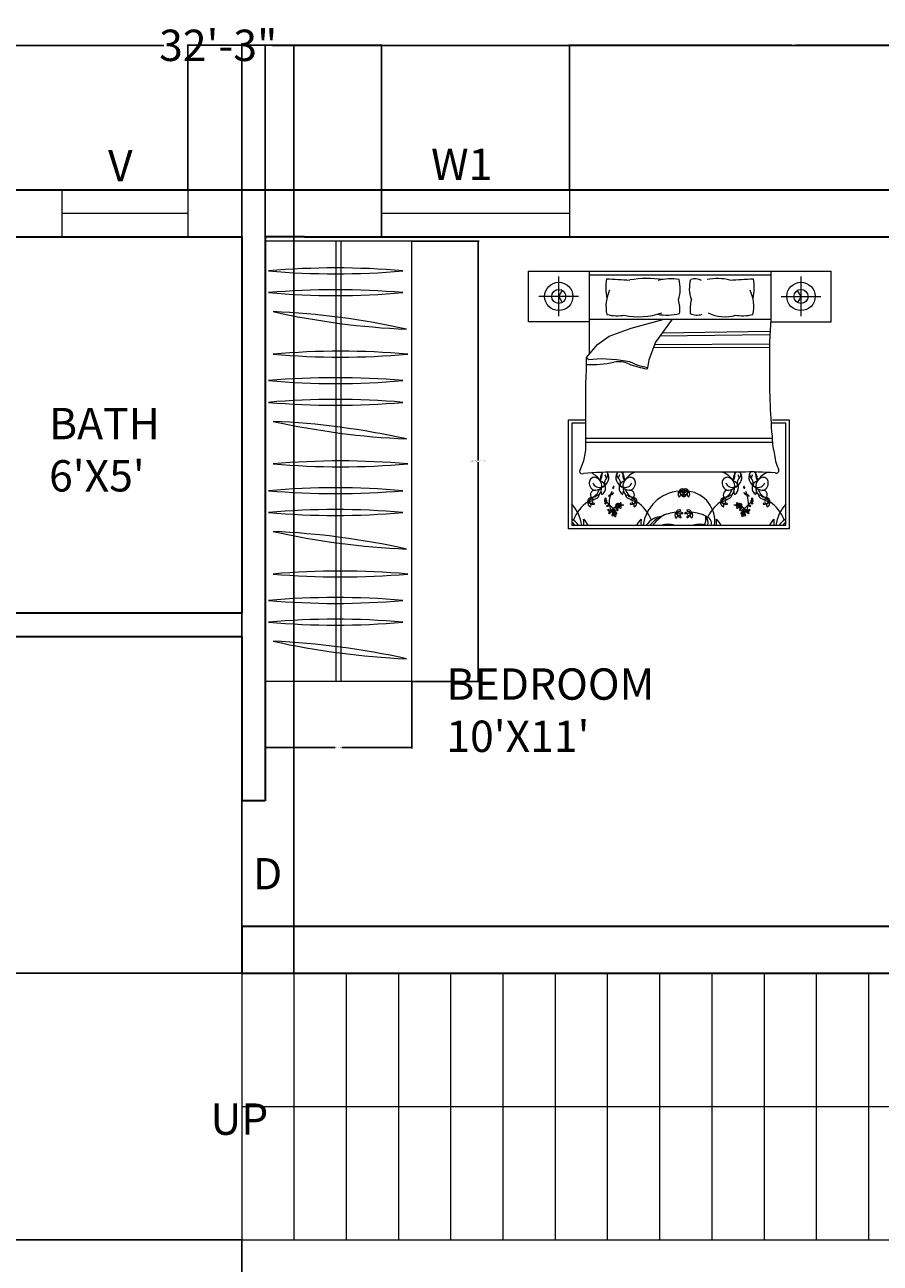
# Model space of a CAD drawing. Units: inches. Extents: x -4347 to -3836, y 955 to 1521.
# Tile 10 of 11: x -4162 to -3998, y 1284 to 1521. Entities that reach past the tile are written whole.
import ezdxf

# ---------------------------------------------------------------- set-up
doc = ezdxf.new("R2010")
doc.units = ezdxf.units.IN
doc.header["$MEASUREMENT"] = 0
for name, color, linetype, lineweight in [('A-ANNO-DIMS', 2, 'Continuous', 18), ('A-ANNO-SYMB', 7, 'Continuous', 18), ('A-ANNO-TEXT', 7, 'Continuous', 18), ('A-AREA-IDEN', 7, 'Continuous', 18), ('A-FLOR-STRS', 7, 'Continuous', 18), ('A-FURN', 8, 'Continuous', 13), ('A-GLAZ', 4, 'Continuous', 18), ('A-WALL', 7, 'Continuous', 35)]:
    doc.layers.add(name, color=color, linetype=linetype, lineweight=lineweight)
doc.styles.get("Standard").update_dxf_attribs({"font": 'arial.ttf'})
doc.dimstyles.get("Standard").update_dxf_attribs({"dimtxt": 0.18, "dimasz": 0.18, "dimexe": 0.18, "dimexo": 0.0625, "dimgap": 0.09, "dimtad": 0, "dimtih": 1, "dimtoh": 1, "dimdec": 0, "dimzin": 0, "dimdsep": 46, "dimlunit": 3, "dimtxsty": 'Standard', "dimcen": 0.09, "dimadec": 0, "dimazin": 0, "dimtfac": 1, "dimtdec": 0, "dimtofl": 0, "dimtmove": 0, "dimatfit": 3, "dimfxl": 1, "dimtolj": 1, "dimtzin": 0, "dimarcsym": 0})

# ---------------------------------------------------------------- blocks, each defined once
blk = doc.blocks.new('*D1')
at = {"layer": 'A-ANNO-DIMS', "color": 0, "lineweight": -2, "transparency": 16777216}
for p, q in [((-4318.58, 1489.85), (-4318.58, 1517.61)), ((-4318.4, 1517.43), (-4135.47, 1517.43)), ((-3931.76, 1517.43), (-4114.69, 1517.43)), ((-3931.58, 1489.85), (-3931.58, 1517.61))]:
    blk.add_line(p, q, dxfattribs=at)
at = {"layer": 'A-ANNO-DIMS', "color": 0, "transparency": 16777216}
for points in [[(-4318.4, 1517.46), (-4318.4, 1517.4), (-4318.58, 1517.43)], [(-3931.76, 1517.46), (-3931.76, 1517.4), (-3931.58, 1517.43)]]:
    blk.add_solid(points, dxfattribs=at)
at = {"layer": 'Defpoints', "color": 0, "transparency": 16777216}
for p in [(-3931.58, 1517.43), (-4318.58, 1489.79), (-3931.58, 1489.79)]:
    blk.add_point(p, dxfattribs=at)
at = {"layer": 'A-ANNO-DIMS', "color": 0, "transparency": 16777216, "insert": (-4125.08, 1517.43), "char_height": 6, "attachment_point": 5}
blk.add_mtext('\\A1;32\'-3"', dxfattribs=at)
blk = doc.blocks.new('BED-DOUBLE-WITH-NIGHTSTANDS')
for p, q in [((0, 49.3), (57.97, 49.3)), ((5.8, 40.68), (5.8, 48.26)), ((11.59, 49.3), (11.59, 33.39)), ((46.38, 48.56), (11.59, 48.56)), ((52.18, 40.68), (52.18, 48.26)), ((9.59, 44.47), (2.01, 44.47)), ((48.39, 44.47), (55.96, 44.47)), ((11.59, 40.14), (46.38, 40.14)), ((15.42, 36.89), (19.65, 38.42)), ((19.65, 38.42), (25.97, 40.14)), ((27.52, 40.14), (24.34, 35.72)), ((13.19, 35.25), (15.42, 36.89)), ((24.34, 35.72), (23.05, 32.32)), ((46.2, 37.14), (25.15, 36.84)), ((46.22, 37.73), (25.58, 37.44)), ((11.08, 32.79), (13.19, 35.25)), ((46.17, 34.72), (23.93, 34.63)), ((46.17, 35.31), (24.16, 35.23)), ((11.55, 32.32), (11.08, 32.79)), ((13.89, 32.55), (11.55, 32.32)), ((16.83, 32.32), (13.89, 32.55)), ((19.41, 31.96), (16.83, 32.32)), ((20.94, 31.26), (19.41, 31.96)), ((22.82, 30.79), (20.94, 31.26)), ((23.05, 32.32), (22.82, 30.79)), ((7.65, 20.88), (10.93, 20.88)), ((7.65, 0), (7.65, 20.88)), ((10.93, 20.21), (8.32, 20.21)), ((8.32, 20.21), (8.32, 0.67)), ((49.25, 20.21), (46.69, 20.21)), ((46.7, 20.88), (49.92, 20.88)), ((49.25, 0.67), (49.25, 20.21)), ((49.92, 20.88), (49.92, 0)), ((46.64, 17.27), (10.93, 17.27)), ((46.7, 16.54), (10.93, 16.54)), ((40.76, 10.85), (17.22, 10.85)), ((14.04, 6.55), (13.91, 7.2)), ((18.09, 6.55), (18.22, 7.2)), ((39.48, 6.55), (39.35, 7.2)), ((43.53, 6.55), (43.66, 7.2)), ((8.32, 0.67), (49.25, 0.67)), ((49.92, 0), (7.65, 0))]:
    blk.add_line(p, q)
for points in [[(11.59, 39.64), (0, 39.64), (0, 49.3)], [(46.38, 49.3), (46.38, 39.64), (57.97, 39.64), (57.97, 49.3)], [(5.8, 44.47), (6.47, 45.64)], [(52.18, 44.47), (51.5, 45.64)], [(5.8, 44.47), (6.47, 43.3)], [(52.18, 44.47), (51.5, 43.3)]]:
    blk.add_lwpolyline(points)
for points in [[(14.92, 47.86, 0.074897), (15, 44.07, -0.472817)], [(28.72, 43.86, 0.14099), (28.83, 47.72, 0.235245)], [(31.19, 43.86, -0.14099), (31.08, 47.72, -0.235245)], [(43.05, 47.86, -0.074897), (42.98, 44.07, 0.472817)], [(10.95, 27.48, 0.001242), (10.93, 16.48, -0.127202), (9.76, 10.99)], [(46.63, 17.72, 0.056112), (47.05, 14.53, 0.095341), (47.86, 11.46)]]:
    blk.add_lwpolyline(points, format="xyb")
for centre, radius in [((5.8, 44.47), 2.71), ((5.8, 44.47), 1.35), ((52.18, 44.47), 2.71), ((52.18, 44.47), 1.35), ((16.42, 2.89), 0.148), ((17.39, 4.45), 0.148), ((40.18, 4.45), 0.148), ((41.15, 2.89), 0.148)]:
    blk.add_circle(centre, radius)
for centre, radius, start, end in [((46.88, 599.58), 552.65, 266.6852, 267.1498), ((22.87, 26.88), 21.03, 82.2196, 99.497), ((27.31, 37.51), 10.33, 81.5249, 103.96), ((31.87, 44.97), 2.87, 63.3437, 106.1026), ((36.17, 37.71), 10.19, 76.3427, 101.1841), ((11.09, 599.58), 552.65, 272.8502, 273.3148), ((22.31, 42.55), 7.47, 155.1316, 191.7583), ((35.66, 42.55), 7.47, 348.2417, 24.8684), ((21.88, 41.92), 7.1, 354.0129, 15.8293), ((38.03, 41.92), 7.1, 164.1707, 185.9871), ((16.99, 48.54), 7.77, 255.1039, 281.0369), ((21.08, 54.06), 13.48, 258.0397, 289.2615), ((26.54, 51.12), 10.22, 259.8617, 283.6238), ((32.26, 43.97), 3.07, 245.0183, 288.5407), ((37.63, 47.96), 7.38, 243.8761, 286.1746), ((40.98, 48.54), 7.77, 258.9631, 284.8961), ((150.31, 33.06), 104.17, 176.1, 180.9282), ((-42.08, 31.34), 53.18, 355.8294, 1.553), ((12.07, 53.32), 21.88, 267.4519, 281.3392), ((17.3, 27.24), 4.72, 66.2616, 101.3392), ((26.84, 52.7), 22.48, 250.1194, 259.3383), ((182.02, 29.27), 135.88, 179.1145, 184.8735), ((22.69, 30.74), 0.14, 268.8623, 19.7536), ((10.3, 11.03), 0.535, 183.98, 297.3412), ((16.53, -49.5), 60.35, 89.3433, 95.6887), ((12.63, 8.87), 0.979, 84.4856, 181.0538), ((10.07, 6.77), 4.39, 33.6671, 63.2997), ((12.33, 8.15), 1.74, 355.2933, 76.921), ((15.95, 9.38), 2.24, 145.785, 184.7304), ((11.68, 10.42), 2.4, 328.8218, 9.1554), ((14.66, 10.21), 0.698, 120.0293, 142.325), ((13.54, 9.8), 1.85, 289.2822, 29.1751), ((15.73, 8.81), 1.19, 131.5653, 195.1471), ((13.26, 9.46), 1.67, 7.436, 29.9149), ((14.36, 10.35), 0.867, 311.5653, 23.8354), ((14.66, 10.21), 0.698, 44.4517, 63.558), ((18.58, 9.8), 1.85, 150.8249, 250.7178), ((17.76, 10.35), 0.867, 156.1646, 228.4347), ((17.47, 10.21), 0.698, 113.229, 135.5483), ((16.4, 8.81), 1.19, 344.8529, 48.4347), ((18.86, 9.46), 1.67, 150.0851, 172.564), ((17.47, 10.21), 0.698, 37.675, 66.7144), ((16.17, 9.38), 2.24, 355.2696, 34.215), ((20.44, 10.42), 2.4, 169.7133, 211.1782), ((19.8, 8.15), 1.74, 103.079, 184.7067), ((22.05, 6.77), 4.39, 111.4941, 146.3329), ((19.5, 8.87), 0.979, 358.9462, 95.5144), ((38.07, 8.87), 0.979, 84.4856, 181.0538), ((35.52, 6.77), 4.39, 33.6671, 68.5059), ((37.77, 8.15), 1.74, 355.2933, 76.921), ((41.4, 9.38), 2.24, 145.785, 184.7304), ((37.13, 10.42), 2.4, 328.8218, 10.2867), ((40.1, 10.21), 0.698, 113.2856, 142.325), ((38.99, 9.8), 1.85, 289.2822, 29.1751), ((41.17, 8.81), 1.19, 131.5653, 195.1471), ((38.71, 9.46), 1.67, 7.436, 29.9149), ((40.1, 10.21), 0.698, 44.4517, 66.7144), ((39.81, 10.35), 0.867, 311.5653, 23.8354), ((42.53, -45.54), 56.41, 85.2402, 91.8035), ((44.03, 9.8), 1.85, 150.8249, 250.7178), ((43.21, 10.35), 0.867, 156.1646, 228.4347), ((42.91, 10.21), 0.698, 106.6343, 135.5483), ((41.84, 8.81), 1.19, 344.8529, 48.4347), ((44.31, 9.46), 1.67, 150.0851, 172.564), ((42.91, 10.21), 0.698, 37.675, 72.5814), ((41.62, 9.38), 2.24, 355.2696, 34.215), ((45.89, 10.42), 2.4, 169.249, 211.1782), ((45.24, 8.15), 1.74, 103.079, 184.7067), ((47.5, 6.77), 4.39, 113.6453, 146.3329), ((44.94, 8.87), 0.979, 358.9462, 95.5144), ((47.42, 11.17), 0.528, 246.5219, 33.8264), ((13.03, 8.73), 1.39, 174.9449, 262.8857), ((12.71, 6.5), 0.87, 80.264, 250.8688), ((13.57, 9.26), 1.35, 201.5819, 291.4221), ((10.99, 8.42), 2.74, 301.2614, 341.7045), ((12.79, 9.04), 1.68, 272.3591, 324.0401), ((10.96, 8.2), 3.11, 326.2883, 356.5076), ((13.32, 7.8), 1.44, 299.9085, 73.1337), ((15.95, 9.38), 2.24, 212.7011, 216.3445), ((14.23, 8.4), 0.36, 257.3041, 15.1471), ((20.25, 4.94), 4.8, 153.0032, 159.8941), ((16.23, 7.86), 0.112, 102.7051, 280.4384), ((16.22, 7.93), 0.182, 280.4384, 100.4136), ((18.81, 7.8), 1.44, 106.8663, 240.0915), ((17.89, 8.4), 0.36, 164.8529, 282.6959), ((16.17, 9.38), 2.24, 323.6555, 327.2989), ((19.34, 9.04), 1.68, 215.9599, 267.6409), ((18.55, 9.26), 1.35, 248.5779, 338.4181), ((21.17, 8.2), 3.11, 183.4924, 213.7117), ((21.14, 8.42), 2.74, 198.2955, 238.7386), ((19.1, 8.73), 1.39, 277.1143, 5.0551), ((19.41, 6.5), 0.87, 289.1312, 99.736), ((29.44, -0.35), 7.57, 94.4623, 172.255), ((29.47, 6.63), 0.84, 137.7873, 219.1145), ((28.52, 6.66), 0.632, 298.5391, 58.3627), ((29.45, 7.02), 0.628, 63.0274, 163.8037), ((28.82, 8.49), 1.29, 271.4585, 315.3727), ((29.34, 6.11), 1.2, 45.5411, 114.3101), ((30.43, 12.25), 5.3, 252.593, 267.2582), ((29.47, 7.17), 0.619, 177.7585, 283.852), ((30.66, 7.82), 1.91, 198.9159, 238.011), ((30.16, 6.11), 1.2, 65.6899, 134.4589), ((29.07, 12.25), 5.3, 272.7418, 287.407), ((30.05, 7.02), 0.628, 16.1963, 116.9726), ((30.69, 8.49), 1.29, 224.6273, 268.5415), ((28.84, 7.82), 1.91, 301.989, 341.0841), ((30.03, 7.17), 0.619, 256.148, 2.2415), ((30.99, 6.66), 0.632, 121.6373, 241.4609), ((30.03, 6.63), 0.84, 320.8855, 42.2127), ((29.82, 1.4), 5.86, 352.8636, 81.8197), ((38.47, 8.73), 1.39, 174.9449, 262.8857), ((38.16, 6.5), 0.87, 80.264, 250.8688), ((39.02, 9.26), 1.35, 201.5819, 291.4221), ((36.43, 8.42), 2.74, 301.2614, 341.7045), ((38.23, 9.04), 1.68, 272.3591, 324.0401), ((36.4, 8.2), 3.11, 326.2883, 356.5076), ((38.76, 7.8), 1.44, 299.9085, 73.1337), ((41.4, 9.38), 2.24, 212.7011, 216.3445), ((39.68, 8.4), 0.36, 257.3041, 15.1471), ((41.35, 7.93), 0.182, 79.5864, 259.5616), ((41.34, 7.86), 0.112, 259.5616, 77.2949), ((37.32, 4.94), 4.8, 20.1059, 26.9968), ((44.25, 7.8), 1.44, 106.8663, 240.0915), ((43.34, 8.4), 0.36, 164.8529, 282.6959), ((41.62, 9.38), 2.24, 323.6555, 327.2989), ((44.78, 9.04), 1.68, 215.9599, 267.6409), ((44, 9.26), 1.35, 248.5779, 338.4181), ((46.61, 8.2), 3.11, 183.4924, 213.7117), ((46.58, 8.42), 2.74, 198.2955, 238.7386), ((44.54, 8.73), 1.39, 277.1143, 5.0551), ((44.86, 6.5), 0.87, 289.1312, 99.736), ((15.64, -1.1), 7.57, 124.3865, 158.5908), ((12.18, 4.97), 0.84, 167.7115, 249.0387), ((11.97, 5.3), 0.628, 92.9516, 193.728), ((10.69, 6.25), 1.29, 301.3827, 345.2969), ((12.34, 4.45), 1.2, 75.4653, 144.2343), ((10.22, 10.32), 5.3, 282.5173, 297.1824), ((11.35, 4.52), 0.632, 328.4633, 88.2869), ((12.62, 6.59), 1.91, 228.8402, 267.9352), ((11.91, 5.44), 0.619, 207.6827, 313.7762), ((12.53, 5.56), 0.533, 63.9755, 143.2681), ((12.28, 5.05), 0.0819, 313.7762, 249.7183), ((12.5, 6.76), 1.09, 265.969, 344.3045), ((12.55, 4.82), 0.0457, 101.4834, 217.9409), ((12.56, 4.77), 0.094, 267.9352, 101.4834), ((13.67, 5.32), 1.16, 96.1662, 141.5825), ((14.73, 5.55), 0.246, 101.5637, 142.6358), ((14.52, 5.33), 0.148, 273.2768, 86.7232), ((14.73, 5.05), 0.244, 217.7621, 259.0403), ((14.7, 5.47), 0.141, 91.1081, 181.8675), ((14.99, 5.38), 0.448, 203.4276, 227.6104), ((14.53, 5.75), 0.355, 288.7263, 352.5032), ((14.85, 5.18), 0.305, 80.3487, 133.6538), ((14.79, 5.43), 0.242, 229.7889, 317.6792), ((14.52, 4.92), 0.343, 355.053, 68.3618), ((14.79, 4.86), 0.483, 83.0852, 105.7171), ((14.77, 5.73), 0.114, 345.2356, 144.9248), ((14.75, 4.9), 0.113, 232.4737, 355.053), ((11.44, 0.86), 5.5, 43.1541, 52.0459), ((14.88, 5.36), 0.127, 317.6792, 80.3487), ((15.59, 6.13), 0.304, 101.3256, 154.4621), ((15.15, 7.16), 0.916, 280.2588, 300.656), ((15.36, 7.9), 1.63, 268.3264, 277.1302), ((20.25, 4.94), 4.8, 163.5842, 183.8277), ((14.95, 7.16), 0.931, 308.2101, 316.3071), ((15.52, 6.55), 0.278, 278.3432, 4.2869), ((15.37, 6.79), 0.486, 300.656, 332.6341), ((15.74, 6.47), 0.118, 55.7657, 157.4417), ((15.92, 6.58), 0.118, 84.3784, 186.0543), ((15.81, 7.06), 0.486, 269.1859, 301.164), ((15.95, 6.81), 0.278, 237.5332, 323.4768), ((15.68, 7.6), 0.931, 285.5129, 293.6099), ((15.59, 7.42), 0.916, 301.164, 321.5612), ((16.29, 6.55), 0.304, 87.3579, 140.4944), ((14.84, 7.58), 1.63, 324.6898, 333.4936), ((16.26, 4.67), 0.673, 304.5369, 16.3699), ((17.19, 4.48), 0.476, 127.3105, 187.9252), ((16.54, 4.53), 0.489, 355.0106, 41.658), ((17.22, 4.65), 0.201, 126.1046, 271.4281), ((17.2, 4.71), 0.145, 353.7526, 131.7054), ((17.59, 4.68), 0.246, 101.5637, 176.365), ((17.39, 4.87), 0.355, 288.7263, 352.5032), ((17.63, 4.85), 0.114, 345.2356, 144.9248), ((18.45, 5.32), 1.16, 38.4175, 83.8338), ((19.62, 6.76), 1.09, 195.6955, 274.031), ((19.59, 5.56), 0.533, 36.7319, 116.0245), ((19.57, 4.77), 0.094, 78.5166, 272.0648), ((19.79, 4.45), 1.2, 35.7657, 104.5347), ((21.91, 10.32), 5.3, 242.8176, 257.4827), ((19.5, 6.59), 1.91, 272.0648, 311.1598), ((19.58, 4.82), 0.0457, 322.0591, 78.5166), ((20.21, 5.44), 0.619, 226.2238, 332.3173), ((19.85, 5.08), 0.0494, 290.2667, 226.2271), ((20.78, 4.52), 0.632, 91.7131, 211.5367), ((20.15, 5.3), 0.628, 346.272, 87.0484), ((21.43, 6.25), 1.29, 194.7031, 238.6173), ((19.94, 4.97), 0.84, 290.9613, 12.2885), ((16.49, -1.1), 7.57, 21.4092, 55.6135), ((29.6, 6.65), 0.0819, 283.852, 219.9245), ((29.7, 6.28), 0.094, 238.011, 71.5592), ((29.71, 6.32), 0.0457, 71.5592, 188.0167), ((29.81, 6.28), 0.094, 108.4408, 301.989), ((29.79, 6.32), 0.0457, 351.9833, 108.4408), ((29.9, 6.68), 0.0494, 320.1909, 256.0209), ((41.08, -1.1), 7.57, 124.3865, 158.5908), ((37.42, 5.3), 0.628, 92.9516, 193.728), ((37.63, 4.97), 0.84, 167.7115, 249.0387), ((36.13, 6.25), 1.29, 301.3827, 345.2969), ((37.78, 4.45), 1.2, 75.4653, 144.2343), ((35.66, 10.32), 5.3, 282.5173, 297.1824), ((37.36, 5.44), 0.619, 207.6827, 313.7762), ((38.07, 6.59), 1.91, 228.8402, 267.9352), ((36.79, 4.52), 0.632, 328.4633, 88.2869), ((37.98, 5.56), 0.533, 63.9755, 143.2681), ((37.73, 5.05), 0.0819, 313.7762, 249.7183), ((37.95, 6.76), 1.09, 265.969, 344.3045), ((37.99, 4.82), 0.0457, 101.4834, 217.9409), ((38, 4.77), 0.094, 267.9352, 101.4834), ((39.12, 5.32), 1.16, 96.1662, 141.5825), ((39.94, 4.85), 0.114, 35.0752, 194.7644), ((40.18, 4.87), 0.355, 187.4968, 251.2737), ((39.98, 4.68), 0.246, 3.635, 78.4363), ((40.37, 4.71), 0.145, 48.2946, 186.2474), ((40.35, 4.65), 0.201, 268.5719, 53.8954), ((41.03, 4.53), 0.489, 138.342, 184.9894), ((41.31, 4.67), 0.673, 163.6301, 235.4631), ((40.38, 4.48), 0.476, 352.0748, 52.6895), ((41.98, 7.42), 0.916, 218.4388, 238.836), ((41.28, 6.55), 0.304, 39.5056, 92.6421), ((42.73, 7.58), 1.63, 206.5064, 215.3102), ((41.62, 6.81), 0.278, 216.5232, 302.4668), ((41.89, 7.6), 0.931, 246.3901, 254.4871), ((41.76, 7.06), 0.486, 238.836, 270.8141), ((41.65, 6.58), 0.118, 353.9457, 95.6216), ((41.83, 6.47), 0.118, 22.5583, 124.2343), ((42.05, 6.55), 0.278, 175.7131, 261.6568), ((42.2, 6.79), 0.486, 207.3659, 239.344), ((37.32, 4.94), 4.8, 356.1723, 16.4158), ((42.62, 7.16), 0.931, 223.6929, 231.7899), ((42.42, 7.16), 0.916, 239.344, 259.7412), ((42.21, 7.9), 1.63, 262.8698, 271.6736), ((41.98, 6.13), 0.304, 25.5379, 78.6744), ((46.13, 0.86), 5.5, 127.9541, 136.8459), ((42.69, 5.36), 0.127, 99.6513, 222.3208), ((42.78, 5.43), 0.242, 222.3208, 310.2111), ((42.72, 5.18), 0.305, 46.3462, 99.6513), ((42.8, 5.73), 0.114, 35.0752, 194.7644), ((43.04, 5.75), 0.355, 187.4968, 251.2737), ((43.05, 4.92), 0.343, 111.6382, 184.947), ((42.82, 4.9), 0.113, 184.947, 307.5263), ((42.78, 4.86), 0.483, 74.2829, 96.9148), ((42.87, 5.47), 0.141, 358.1325, 88.8919), ((42.58, 5.38), 0.448, 312.3896, 336.5724), ((42.84, 5.55), 0.246, 37.3642, 78.4363), ((42.84, 5.05), 0.244, 280.9597, 322.2379), ((43.05, 5.33), 0.148, 93.2768, 266.7232), ((45.07, 6.76), 1.09, 195.6955, 274.031), ((43.9, 5.32), 1.16, 38.4175, 83.8338), ((45.04, 5.56), 0.533, 36.7319, 116.0245), ((45.01, 4.77), 0.094, 78.5166, 272.0648), ((45.23, 4.45), 1.2, 35.7657, 104.5347), ((47.35, 10.32), 5.3, 242.8176, 257.4827), ((44.95, 6.59), 1.91, 272.0648, 311.1598), ((45.02, 4.82), 0.0457, 322.0591, 78.5166), ((45.66, 5.44), 0.619, 226.2238, 332.3173), ((45.29, 5.08), 0.0494, 290.2667, 226.2271), ((46.22, 4.52), 0.632, 91.7131, 211.5367), ((46.88, 6.25), 1.29, 194.7031, 238.6173), ((45.6, 5.3), 0.628, 346.272, 87.0484), ((45.39, 4.97), 0.84, 290.9613, 12.2885), ((41.93, -1.1), 7.57, 21.4092, 55.6135), ((2.69, -0.35), 7.57, 7.745, 41.8856), ((15.24, 4.18), 0.304, 101.3256, 154.4621), ((14.81, 5.21), 0.916, 280.2588, 300.656), ((15.02, 5.95), 1.63, 268.3264, 277.1302), ((14.61, 5.21), 0.931, 308.2101, 316.3071), ((15.35, 3.65), 0.165, 146.8636, 236.9021), ((17.67, 7.28), 4.31, 235.1882, 238.8844), ((15.63, 3.89), 0.446, 199.4799, 267.6828), ((15.18, 4.6), 0.278, 278.3432, 4.2869), ((15.58, 3.72), 0.384, 212.8155, 277.3992), ((15.03, 4.84), 0.486, 300.656, 332.6341), ((15.39, 4.52), 0.118, 55.7657, 157.4417), ((15.36, 3.46), 0.446, 266.9701, 338.2913), ((13, 6.64), 4.31, 302.6784, 306.3746), ((15.47, 3.11), 0.165, 214.3538, 304.3923), ((15.53, 3.73), 0.171, 238.8844, 314.2646), ((17.86, 4.82), 2.41, 184.756, 209.2041), ((21.32, 9.95), 7.92, 222.2412, 232.1744), ((15.49, 3.35), 0.384, 280.3057, 17.1958), ((15.46, 3.31), 0.171, 306.3746, 21.7548), ((15.74, 3.42), 0.129, 19.3605, 201.7548), ((15.74, 3.52), 0.129, 311.8703, 134.2646), ((18.16, 2.34), 2.57, 153.7819, 158.2913), ((16.11, 4.1), 0.673, 247.2305, 319.0635), ((15.89, 3.87), 0.396, 264.4544, 310.6188), ((17.86, 4.82), 2.41, 214.0033, 222.4917), ((16.18, 3.72), 0.409, 218.3208, 298.8162), ((18.1, 1.62), 2.89, 120.544, 139.818), ((16.11, 2.62), 0.146, 148.0499, 225.6268), ((16.38, 2.45), 0.465, 104.7558, 148.0499), ((16.12, 2.78), 0.291, 247.4086, 351.4386), ((16.26, 3.1), 0.201, 126.1046, 271.4281), ((16.24, 3.15), 0.145, 353.7526, 131.7054), ((16.46, 3.21), 0.476, 70.0041, 130.6188), ((16.2, 2.77), 0.0978, 262.906, 7.132), ((16.1, 2.98), 0.203, 0.0645, 61.1507), ((16.15, 3.15), 0.232, 311.8413, 355.7877), ((16.15, 3.79), 0.489, 297.7043, 344.3516), ((16.62, 3.12), 0.246, 101.5637, 176.365), ((16.62, 2.62), 0.244, 151.2196, 259.0403), ((16.59, 3.03), 0.141, 91.1081, 181.8675), ((16.88, 2.94), 0.448, 203.4276, 227.6104), ((16.74, 2.75), 0.305, 80.3487, 133.6538), ((16.69, 3), 0.242, 229.7889, 317.6792), ((16.43, 3.31), 0.355, 288.7263, 352.5032), ((16.42, 2.49), 0.343, 355.053, 68.3618), ((16.68, 2.43), 0.483, 83.0852, 105.7171), ((16.67, 3.3), 0.114, 345.2356, 144.9248), ((16.64, 2.47), 0.113, 232.4737, 355.053), ((16.62, 4.52), 0.409, 272.8499, 356.1226), ((16.33, 4.36), 0.396, 321.7607, 7.9252), ((16.41, 3.79), 0.396, 8.7227, 54.8872), ((16.43, 3.47), 0.673, 0.278, 72.111), ((16.73, 3.72), 0.409, 20.5253, 88.5375), ((16.77, 2.92), 0.127, 317.6792, 80.3487), ((17.27, 3.92), 0.476, 188.7227, 249.3375), ((17.08, 4.17), 0.146, 148.0499, 225.6268), ((18.1, 1.62), 2.89, 113.0501, 113.8477), ((17.35, 4), 0.465, 104.7558, 148.0499), ((17.09, 4.34), 0.291, 247.4086, 351.4386), ((16.66, 3.68), 0.489, 334.9899, 21.6373), ((17.06, 4.54), 0.203, 0.0645, 61.1507), ((17.17, 4.32), 0.0978, 262.906, 7.132), ((17.11, 4.71), 0.232, 311.8413, 355.7877), ((17.59, 4.18), 0.244, 151.2196, 259.0403), ((17.56, 4.59), 0.141, 91.1081, 181.8675), ((17.85, 4.5), 0.448, 203.4276, 227.6104), ((17.71, 4.3), 0.305, 80.3487, 133.6538), ((17.65, 4.56), 0.242, 229.7889, 317.6792), ((17.38, 4.05), 0.343, 355.053, 68.3618), ((17.65, 3.99), 0.483, 83.0852, 105.7171), ((17.61, 4.03), 0.113, 232.4737, 355.053), ((17.74, 4.48), 0.127, 317.6792, 80.3487), ((18.1, 1.62), 2.89, 87.1071, 94.7585), ((28.86, -4.4), 7.57, 94.4623, 117.4146), ((28.89, 2.58), 0.84, 137.7873, 219.1145), ((27.94, 2.61), 0.632, 298.5391, 58.3627), ((28.87, 2.97), 0.628, 63.0274, 163.8037), ((28.24, 4.44), 1.29, 271.4585, 315.3727), ((28.76, 2.05), 1.2, 45.5411, 114.3101), ((30.08, 3.76), 1.91, 198.9159, 238.011), ((29.85, 8.2), 5.3, 252.593, 267.2582), ((28.89, 3.12), 0.619, 177.7585, 283.852), ((29.02, 2.6), 0.0819, 283.852, 219.9245), ((30.74, 2.05), 1.2, 65.6899, 134.4589), ((29.65, 8.2), 5.3, 272.7418, 287.407), ((30.63, 2.97), 0.628, 16.1963, 116.9726), ((31.27, 4.44), 1.29, 224.6273, 268.5415), ((30.48, 2.63), 0.0494, 320.1909, 256.0209), ((29.42, 3.76), 1.91, 301.989, 341.0841), ((30.61, 3.12), 0.619, 256.148, 2.2415), ((31.56, 2.61), 0.632, 121.6373, 241.4609), ((30.61, 2.58), 0.84, 320.8855, 42.2127), ((30.64, -4.4), 7.57, 62.5854, 85.5377), ((39.47, 1.62), 2.89, 85.2415, 92.8929), ((39.83, 4.48), 0.127, 99.6513, 222.3208), ((39.92, 4.56), 0.242, 222.3208, 310.2111), ((39.86, 4.3), 0.305, 46.3462, 99.6513), ((40.19, 4.05), 0.343, 111.6382, 184.947), ((39.96, 4.03), 0.113, 184.947, 307.5263), ((39.92, 3.99), 0.483, 74.2829, 96.9148), ((40.01, 4.59), 0.141, 358.1325, 88.8919), ((39.72, 4.5), 0.448, 312.3896, 336.5724), ((39.98, 4.18), 0.244, 280.9597, 28.7804), ((40.48, 4.34), 0.291, 188.5614, 292.5914), ((40.46, 4.71), 0.232, 184.2123, 228.1587), ((40.5, 4.54), 0.203, 118.8493, 179.9355), ((40.4, 4.32), 0.0978, 172.868, 277.094), ((40.22, 4), 0.465, 31.9501, 75.2442), ((40.91, 3.68), 0.489, 158.3627, 205.0101), ((40.84, 3.72), 0.409, 91.4625, 159.4747), ((41.14, 3.47), 0.673, 107.889, 179.722), ((40.3, 3.92), 0.476, 290.6625, 351.2773), ((40.95, 4.52), 0.409, 183.8774, 267.1501), ((39.47, 1.62), 2.89, 66.1523, 66.9499), ((40.49, 4.17), 0.146, 314.3732, 31.9501), ((40.8, 2.92), 0.127, 99.6513, 222.3208), ((40.88, 3), 0.242, 222.3208, 310.2111), ((41.16, 3.79), 0.396, 125.1128, 171.2773), ((40.83, 2.75), 0.305, 46.3462, 99.6513), ((40.9, 3.3), 0.114, 35.0752, 194.7644), ((41.14, 3.31), 0.355, 187.4968, 251.2737), ((41.15, 2.49), 0.343, 111.6382, 184.947), ((40.93, 2.47), 0.113, 184.947, 307.5263), ((40.89, 2.43), 0.483, 74.2829, 96.9148), ((41.24, 4.36), 0.396, 172.0748, 218.2393), ((39.47, 1.62), 2.89, 40.182, 59.456), ((41.11, 3.21), 0.476, 49.3812, 109.9959), ((41.46, 4.1), 0.673, 220.9365, 292.7695), ((41.42, 3.79), 0.489, 195.6484, 242.2957), ((40.98, 3.03), 0.141, 358.1325, 88.8919), ((40.95, 3.12), 0.246, 3.635, 78.4363), ((40.68, 2.94), 0.448, 312.3896, 336.5724), ((40.95, 2.62), 0.244, 280.9597, 28.7804), ((36.25, 9.95), 7.92, 307.8256, 317.7588), ((41.45, 2.78), 0.291, 188.5614, 292.5914), ((41.39, 3.72), 0.409, 241.1838, 321.6792), ((41.33, 3.15), 0.145, 48.2946, 186.2474), ((41.42, 3.15), 0.232, 184.2123, 228.1587), ((41.47, 2.98), 0.203, 118.8493, 179.9355), ((41.37, 2.77), 0.0978, 172.868, 277.094), ((41.31, 3.1), 0.201, 268.5719, 53.8954), ((41.19, 2.45), 0.465, 31.9501, 75.2442), ((41.68, 3.87), 0.396, 229.3812, 275.5456), ((39.71, 4.82), 2.41, 317.5083, 325.9967), ((41.46, 2.62), 0.146, 314.3732, 31.9501), ((42.08, 3.35), 0.384, 162.8042, 259.6943), ((41.83, 3.52), 0.129, 45.7354, 228.1297), ((41.83, 3.42), 0.129, 338.2452, 160.6395), ((39.41, 2.34), 2.57, 21.7087, 26.2181), ((42.21, 3.46), 0.446, 201.7087, 273.0299), ((39.71, 4.82), 2.41, 330.7959, 355.244), ((42.04, 3.73), 0.171, 225.7354, 301.1156), ((41.99, 3.72), 0.384, 262.6008, 327.1845), ((42.11, 3.31), 0.171, 158.2452, 233.6254), ((41.94, 3.89), 0.446, 272.3172, 340.5201), ((44.57, 6.64), 4.31, 233.6254, 237.3216), ((42.1, 3.11), 0.165, 235.6077, 325.6462), ((42.18, 4.52), 0.118, 22.5583, 124.2343), ((42.39, 4.6), 0.278, 175.7131, 261.6568), ((42.54, 4.84), 0.486, 207.3659, 239.344), ((39.9, 7.28), 4.31, 301.1156, 304.8118), ((42.96, 5.21), 0.931, 223.6929, 231.7899), ((42.76, 5.21), 0.916, 239.344, 259.7412), ((42.22, 3.65), 0.165, 303.0979, 33.1364), ((42.55, 5.95), 1.63, 262.8698, 271.6736), ((42.33, 4.18), 0.304, 25.5379, 78.6744), ((54.88, -0.35), 7.57, 138.1144, 172.255), ((6.49, -1.36), 3.69, 33.4617, 60.1116), ((5.16, -2.05), 4.6, 36.3036, 46.4814), ((8.55, -0.51), 3.08, 22.5547, 48.9546), ((0.12, 1.15), 10.47, 357.4081, 3.6519), ((23.57, -0.51), 3.08, 131.0454, 157.4453), ((32.01, 1.15), 10.47, 176.3481, 182.5919), ((25.64, -1.36), 3.69, 91.272, 146.5383), ((26.97, -2.05), 4.6, 107.8504, 143.6964), ((29.38, -3.34), 6.84, 124.0123, 144.053), ((26.74, -3.31), 4.16, 73.5431, 107.0202), ((28.39, -5.45), 6.16, 94.3787, 95.6357), ((31.63, -9.67), 11, 109.7217, 109.9028), ((29.12, 2.22), 0.094, 238.011, 71.5592), ((29.13, 2.27), 0.0457, 71.5592, 188.0167), ((30.39, 2.22), 0.094, 108.4408, 301.989), ((30.37, 2.27), 0.0457, 351.9833, 108.4408), ((32.76, -3.31), 4.16, 72.9798, 106.4569), ((31.11, -5.45), 6.16, 84.3643, 85.6213), ((27.87, -9.67), 11, 70.0972, 70.2783), ((30.58, 1.93), 3.39, 338.117, 6.6195), ((33.69, 0.99), 1.36, 346.3898, 79.0739), ((32.67, 1.18), 1.72, 342.8609, 41.9049), ((25.56, 1.15), 10.47, 357.4081, 3.6519), ((34, -0.51), 3.08, 22.5547, 48.9546), ((49.02, -0.51), 3.08, 131.0454, 157.4453), ((57.45, 1.15), 10.47, 176.3481, 182.5919), ((51.08, -1.36), 3.69, 119.8884, 146.5383), ((52.41, -2.05), 4.6, 133.5186, 143.6964)]:
    blk.add_arc(centre, radius, start, end)
blk = doc.blocks.new('WARDROBE-LONG')
for p, q in [((0, 0), (0, 84.3)), ((28.1, 84.3), (0, 84.3)), ((13.58, 0), (13.58, 84.3)), ((14.52, 0), (14.52, 84.3)), ((28.1, 0), (28.1, 84.3)), ((28.1, 0), (0, 0))]:
    blk.add_line(p, q)
for centre, start, end in [((13.49, -68.71), 85.0028, 94.9972), ((13.49, 225.88), 265.0028, 274.9972), ((13.49, -72.88), 85.0028, 94.9972), ((13.49, 221.72), 265.0028, 274.9972), ((33.49, 215.14), 257.508, 267.5023), ((-4.93, -76.94), 77.508, 87.5023), ((14.4, -84.65), 85.0028, 94.9972), ((14.4, 209.94), 265.0028, 274.9972), ((13.49, -89.72), 85.0028, 94.9972), ((13.49, 204.88), 265.0028, 274.9972), ((13.49, -93.88), 85.0028, 94.9972), ((13.49, 200.71), 265.0028, 274.9972), ((33.49, 194.14), 257.508, 267.5023), ((-4.93, -97.94), 77.508, 87.5023), ((14.4, -105.66), 85.0028, 94.9972), ((14.4, 188.94), 265.0028, 274.9972), ((13.49, -110.8), 85.0028, 94.9972), ((13.49, 183.8), 265.0028, 274.9972), ((13.49, -114.96), 85.0028, 94.9972), ((13.49, 179.63), 265.0028, 274.9972), ((-4.93, -119.02), 77.508, 87.5023), ((33.49, 173.05), 257.508, 267.5023), ((14.4, -126.74), 85.0028, 94.9972), ((14.4, 167.85), 265.0028, 274.9972), ((13.49, -131.8), 85.0028, 94.9972), ((13.49, 162.79), 265.0028, 274.9972), ((13.49, -135.96), 85.0028, 94.9972), ((13.49, 158.63), 265.0028, 274.9972), ((-4.93, -140.03), 77.508, 87.5023), ((33.49, 152.05), 257.508, 267.5023)]:
    blk.add_arc(centre, 147.86, start, end)
blk = doc.blocks.new('GLAZ-24IN')
for p, q in [((0, 9), (24, 9)), ((0, 0), (0, 9)), ((24, 9), (24, 0)), ((0, 4.5), (24, 4.5)), ((24, 0), (0, 0))]:
    blk.add_line(p, q)
blk = doc.blocks.new('*D16')
at = {"layer": 'A-ANNO-DIMS', "color": 0, "lineweight": -2, "transparency": 16777216}
for p, q in [((-4087.92, 1479.97), (-4075.15, 1479.97)), ((-4075.33, 1479.79), (-4075.33, 1438.01)), ((-4075.33, 1395.85), (-4075.33, 1437.64)), ((-4087.92, 1395.67), (-4075.15, 1395.67))]:
    blk.add_line(p, q, dxfattribs=at)
at = {"layer": 'A-ANNO-DIMS', "color": 0, "transparency": 16777216}
for points in [[(-4075.36, 1479.79), (-4075.3, 1479.79), (-4075.33, 1479.97)], [(-4075.36, 1395.85), (-4075.3, 1395.85), (-4075.33, 1395.67)]]:
    blk.add_solid(points, dxfattribs=at)
at = {"layer": 'Defpoints', "color": 0, "transparency": 16777216}
for p in [(-4087.98, 1479.97), (-4075.33, 1479.97), (-4087.98, 1395.67)]:
    blk.add_point(p, dxfattribs=at)
at = {"layer": 'A-ANNO-DIMS', "color": 0, "transparency": 16777216, "insert": (-4075.33, 1437.82), "char_height": 0.18, "attachment_point": 5}
blk.add_mtext('\\A1;WARDROBE 7\'-0 1/2" TYP.', dxfattribs=at)
blk = doc.blocks.new('*D17')
at = {"layer": 'A-ANNO-DIMS', "color": 0, "lineweight": -2, "transparency": 16777216}
for p, q in [((-4116.08, 1395.61), (-4116.08, 1382.85)), ((-4087.98, 1395.61), (-4087.98, 1382.85)), ((-4115.9, 1383.03), (-4102.67, 1383.03)), ((-4088.16, 1383.03), (-4101.39, 1383.03))]:
    blk.add_line(p, q, dxfattribs=at)
at = {"layer": 'A-ANNO-DIMS', "color": 0, "transparency": 16777216}
for points in [[(-4115.9, 1383.06), (-4115.9, 1383), (-4116.08, 1383.03)], [(-4088.16, 1383.06), (-4088.16, 1383), (-4087.98, 1383.03)]]:
    blk.add_solid(points, dxfattribs=at)
at = {"layer": 'Defpoints', "color": 0, "transparency": 16777216}
for p in [(-4116.08, 1395.67), (-4087.98, 1395.67), (-4087.98, 1383.03)]:
    blk.add_point(p, dxfattribs=at)
at = {"layer": 'A-ANNO-DIMS', "color": 0, "transparency": 16777216, "insert": (-4102.03, 1383.03), "char_height": 0.18, "attachment_point": 5}
blk.add_mtext('\\A1;2\'-4" TYP.', dxfattribs=at)
blk = doc.blocks.new('*D36')
at = {"layer": 'A-ANNO-DIMS', "color": 0, "lineweight": -2, "transparency": 16777216}
for p, q in [((-4130.93, 1489.85), (-4130.93, 1517.62)), ((-4130.75, 1517.44), (-4112.69, 1517.44)), ((-4093.98, 1517.44), (-4112.03, 1517.44)), ((-4093.8, 1489.85), (-4093.8, 1517.62))]:
    blk.add_line(p, q, dxfattribs=at)
at = {"layer": 'A-ANNO-DIMS', "color": 0, "transparency": 16777216}
for points in [[(-4130.75, 1517.47), (-4130.75, 1517.41), (-4130.93, 1517.44)], [(-4093.98, 1517.47), (-4093.98, 1517.41), (-4093.8, 1517.44)]]:
    blk.add_solid(points, dxfattribs=at)
at = {"layer": 'Defpoints', "color": 0, "transparency": 16777216}
for p in [(-4093.8, 1517.44), (-4130.93, 1489.79), (-4093.8, 1489.79)]:
    blk.add_point(p, dxfattribs=at)
at = {"layer": 'A-ANNO-DIMS', "color": 0, "transparency": 16777216, "insert": (-4112.36, 1517.44), "char_height": 0.18, "attachment_point": 5}
blk.add_mtext('\\A1;3\'-1"', dxfattribs=at)
blk = doc.blocks.new('*D37')
at = {"layer": 'A-ANNO-DIMS', "color": 0, "lineweight": -2, "transparency": 16777216}
for p, q in [((-4116.08, 1480.85), (-4116.08, 1517.62)), ((-4115.9, 1517.44), (-4105.54, 1517.44)), ((-4093.98, 1517.44), (-4104.34, 1517.44)), ((-4093.8, 1480.85), (-4093.8, 1517.62))]:
    blk.add_line(p, q, dxfattribs=at)
at = {"layer": 'A-ANNO-DIMS', "color": 0, "transparency": 16777216}
for points in [[(-4115.9, 1517.47), (-4115.9, 1517.41), (-4116.08, 1517.44)], [(-4093.98, 1517.47), (-4093.98, 1517.41), (-4093.8, 1517.44)]]:
    blk.add_solid(points, dxfattribs=at)
at = {"layer": 'Defpoints', "color": 0, "transparency": 16777216}
for p in [(-4093.8, 1517.44), (-4116.08, 1480.79), (-4093.8, 1480.79)]:
    blk.add_point(p, dxfattribs=at)
at = {"layer": 'A-ANNO-DIMS', "color": 0, "transparency": 16777216, "insert": (-4104.94, 1517.44), "char_height": 0.18, "attachment_point": 5}
blk.add_mtext('\\A1;1\'-10 1/2"', dxfattribs=at)
blk = doc.blocks.new('*D38')
at = {"layer": 'A-ANNO-DIMS', "color": 0, "lineweight": -2, "transparency": 16777216}
for p, q in [((-4057.8, 1489.85), (-4057.8, 1517.62)), ((-4057.62, 1517.44), (-4015.23, 1517.44)), ((-3972.19, 1517.44), (-4014.57, 1517.44)), ((-3972.01, 1489.85), (-3972.01, 1517.62))]:
    blk.add_line(p, q, dxfattribs=at)
at = {"layer": 'A-ANNO-DIMS', "color": 0, "transparency": 16777216}
for points in [[(-4057.62, 1517.47), (-4057.62, 1517.41), (-4057.8, 1517.44)], [(-3972.19, 1517.47), (-3972.19, 1517.41), (-3972.01, 1517.44)]]:
    blk.add_solid(points, dxfattribs=at)
at = {"layer": 'Defpoints', "color": 0, "transparency": 16777216}
for p in [(-3972.01, 1517.44), (-4057.8, 1489.79), (-3972.01, 1489.79)]:
    blk.add_point(p, dxfattribs=at)
at = {"layer": 'A-ANNO-DIMS', "color": 0, "transparency": 16777216, "insert": (-4014.9, 1517.44), "char_height": 0.18, "attachment_point": 5}
blk.add_mtext('\\A1;7\'-2"', dxfattribs=at)
blk = doc.blocks.new('*D47')
at = {"layer": 'A-ANNO-DIMS', "color": 0, "lineweight": -2, "transparency": 16777216}
for p, q in [((-4120.58, 1288.73), (-4120.58, 966.96)), ((-3940.58, 1288.73), (-3940.58, 966.96)), ((-4120.4, 967.14), (-4030.97, 967.14)), ((-3940.76, 967.14), (-4030.19, 967.14))]:
    blk.add_line(p, q, dxfattribs=at)
at = {"layer": 'A-ANNO-DIMS', "color": 0, "transparency": 16777216}
for points in [[(-4120.4, 967.17), (-4120.4, 967.11), (-4120.58, 967.14)], [(-3940.76, 967.17), (-3940.76, 967.11), (-3940.58, 967.14)]]:
    blk.add_solid(points, dxfattribs=at)
at = {"layer": 'Defpoints', "color": 0, "transparency": 16777216}
for p in [(-4120.58, 1288.79), (-3940.58, 1288.79), (-3940.58, 967.14)]:
    blk.add_point(p, dxfattribs=at)
at = {"layer": 'A-ANNO-DIMS', "color": 0, "transparency": 16777216, "insert": (-4030.58, 967.14), "char_height": 0.18, "attachment_point": 5}
blk.add_mtext('\\A1;15\'-0"', dxfattribs=at)
blk = doc.blocks.new('*D48')
at = {"layer": 'A-ANNO-DIMS', "color": 0, "lineweight": -2, "transparency": 16777216}
for p, q in [((-4120.64, 1339.79), (-4346.41, 1339.79)), ((-4346.23, 1339.61), (-4346.23, 1314.47)), ((-4346.23, 1288.97), (-4346.23, 1314.11)), ((-4120.64, 1288.79), (-4346.41, 1288.79))]:
    blk.add_line(p, q, dxfattribs=at)
at = {"layer": 'A-ANNO-DIMS', "color": 0, "transparency": 16777216}
for points in [[(-4346.26, 1339.61), (-4346.2, 1339.61), (-4346.23, 1339.79)], [(-4346.26, 1288.97), (-4346.2, 1288.97), (-4346.23, 1288.79)]]:
    blk.add_solid(points, dxfattribs=at)
at = {"layer": 'Defpoints', "color": 0, "transparency": 16777216}
for p in [(-4346.23, 1339.79), (-4120.58, 1339.79), (-4120.58, 1288.79)]:
    blk.add_point(p, dxfattribs=at)
at = {"layer": 'A-ANNO-DIMS', "color": 0, "transparency": 16777216, "insert": (-4346.23, 1314.29), "char_height": 0.18, "attachment_point": 5}
blk.add_mtext('\\A1;4\'-3"', dxfattribs=at)
blk = doc.blocks.new('*D49')
at = {"layer": 'A-ANNO-DIMS', "color": 0, "lineweight": -2, "transparency": 16777216}
for p, q in [((-4120.58, 1339.85), (-4120.58, 1517.62)), ((-4120.4, 1517.44), (-4115.98, 1517.44)), ((-4110.76, 1517.44), (-4115.18, 1517.44)), ((-4110.58, 1339.85), (-4110.58, 1517.62))]:
    blk.add_line(p, q, dxfattribs=at)
at = {"layer": 'A-ANNO-DIMS', "color": 0, "transparency": 16777216}
for points in [[(-4120.4, 1517.47), (-4120.4, 1517.41), (-4120.58, 1517.44)], [(-4110.76, 1517.47), (-4110.76, 1517.41), (-4110.58, 1517.44)]]:
    blk.add_solid(points, dxfattribs=at)
at = {"layer": 'Defpoints', "color": 0, "transparency": 16777216}
for p in [(-4110.58, 1517.44), (-4120.58, 1339.79), (-4110.58, 1339.79)]:
    blk.add_point(p, dxfattribs=at)
at = {"layer": 'A-ANNO-DIMS', "color": 0, "transparency": 16777216, "insert": (-4115.58, 1517.44), "char_height": 0.18, "attachment_point": 5}
blk.add_mtext('\\A1;0\'-10"', dxfattribs=at)

msp = doc.modelspace()

# ---------------------------------------------------------------- linework, layer by layer
at = {"layer": 'A-ANNO-SYMB'}
msp.add_line((-4120.58, 1314.29), (-3963.77, 1314.29), dxfattribs=at)
at = {"layer": 'A-FLOR-STRS'}
for p, q in [((-4120.58, 1339.79), (-4120.58, 1288.79)), ((-4110.58, 1339.79), (-4110.58, 1288.79)), ((-4100.58, 1339.79), (-4100.58, 1288.79)), ((-4090.58, 1339.79), (-4090.58, 1288.79)), ((-4080.58, 1339.79), (-4080.58, 1288.79)), ((-4070.58, 1339.79), (-4070.58, 1288.79)), ((-4060.58, 1339.79), (-4060.58, 1288.79)), ((-4050.58, 1339.79), (-4050.58, 1288.79)), ((-4040.58, 1339.79), (-4040.58, 1288.79)), ((-4030.58, 1339.79), (-4030.58, 1288.79)), ((-4020.58, 1339.79), (-4020.58, 1288.79)), ((-4010.58, 1339.79), (-4010.58, 1288.79)), ((-4000.58, 1339.79), (-4000.58, 1288.79)), ((-4120.58, 1288.79), (-3940.58, 1288.79))]:
    msp.add_line(p, q, dxfattribs=at)
at = {"layer": 'A-GLAZ'}
for p, q in [((-4093.8, 1489.79), (-4057.8, 1489.79)), ((-4093.8, 1480.79), (-4093.8, 1489.79)), ((-4057.8, 1489.79), (-4057.8, 1480.79)), ((-4093.8, 1485.29), (-4057.8, 1485.29)), ((-4081.8, 1480.79), (-4093.8, 1480.79)), ((-4057.8, 1480.79), (-4081.8, 1480.79))]:
    msp.add_line(p, q, dxfattribs=at)
at = {"layer": 'A-WALL'}
for p, q in [((-4318.58, 1489.79), (-3931.58, 1489.79)), ((-4185.08, 1480.79), (-4120.58, 1480.79)), ((-4120.58, 1480.79), (-4120.58, 1408.79)), ((-4108.58, 1480.79), (-4116.08, 1480.79)), ((-4116.08, 1480.79), (-4116.08, 1372.79)), ((-4108.58, 1480.79), (-3996.08, 1480.79)), ((-4189.58, 1408.79), (-4120.58, 1408.79)), ((-4185.08, 1404.29), (-4120.58, 1404.29)), ((-4120.58, 1404.29), (-4120.58, 1372.79)), ((-4116.08, 1372.79), (-4120.58, 1372.79)), ((-4120.58, 1348.79), (-3996.08, 1348.79)), ((-4120.58, 1348.79), (-4120.58, 1339.79)), ((-4120.58, 1339.79), (-3940.58, 1339.79))]:
    msp.add_line(p, q, dxfattribs=at)

# ---------------------------------------------------------------- block references
at = {"layer": 'A-FURN'}
for name, p in [('WARDROBE-LONG', (-4116.08, 1395.67)), ('BED-DOUBLE-WITH-NIGHTSTANDS', (-4065.68, 1424.89))]:
    msp.add_blockref(name, p, dxfattribs=at)
at = {"layer": 'A-GLAZ'}
msp.add_blockref('GLAZ-24IN', (-4154.93, 1480.79), dxfattribs=at)

# ---------------------------------------------------------------- texts
at = {"layer": 'A-ANNO-SYMB', "insert": (-4126.58, 1314.88), "char_height": 6, "attachment_point": 1}
msp.add_mtext('UP', dxfattribs=at)
at = {"layer": 'A-ANNO-TEXT', "char_height": 6, "attachment_point": 1}
for s, insert in [('V', (-4146.18, 1497.4)), ('D', (-4118.45, 1361.85))]:
    msp.add_mtext(s, dxfattribs=dict(at, insert=insert))
at = {"layer": 'A-ANNO-TEXT', "insert": (-4084.33, 1497.66), "char_height": 6, "attachment_point": 1}
msp.add_mtext_dynamic_manual_height_columns('W1', width=0.1196, gutter_width=1, heights=[0], dxfattribs=at)
at = {"layer": 'A-AREA-IDEN', "insert": (-4157.47, 1448.02), "char_height": 6, "attachment_point": 1}
msp.add_mtext("BATH\\P6'X5'", dxfattribs=at)
at = {"layer": 'A-AREA-IDEN', "insert": (-4081.41, 1398.16), "char_height": 6, "attachment_point": 1}
msp.add_mtext_dynamic_manual_height_columns("BEDROOM\\P10'X11'", width=0.6153, gutter_width=1, heights=[0], dxfattribs=at)

# ---------------------------------------------------------------- dimensions: what is measured, and where the dimension line sits
at = {"layer": 'A-ANNO-DIMS'}
for base, p1, p2, override, picture, middle in [((-3931.58, 1517.43), (-4318.58, 1489.79), (-3931.58, 1489.79), {"dimtxt": 6, "dimclrd": 0, "dimclre": 0, "dimclrt": 0}, '*D1', (-4125.08, 1517.43)), ((-4093.8, 1517.44), (-4130.93, 1489.79), (-4093.8, 1489.79), {"dimdec": 1, "dimlfac": 1, "dimrnd": 0, "dimzin": 1, "dimdsep": 46, "dimlunit": 4, "dimfrac": 2}, '*D36', (-4112.36, 1517.44)), ((-4110.58, 1517.44), (-4120.58, 1339.79), (-4110.58, 1339.79), {"dimdec": 1, "dimlfac": 1, "dimrnd": 0, "dimzin": 1, "dimdsep": 46, "dimlunit": 4, "dimfrac": 2}, '*D49', (-4115.58, 1517.44)), ((-4093.8, 1517.44), (-4116.08, 1480.79), (-4093.8, 1480.79), {"dimdec": 1, "dimlfac": 1, "dimrnd": 0, "dimzin": 1, "dimdsep": 46, "dimlunit": 4, "dimfrac": 2}, '*D37', (-4104.94, 1517.44)), ((-3972.01, 1517.44), (-4057.8, 1489.79), (-3972.01, 1489.79), {"dimdec": 1, "dimlfac": 1, "dimrnd": 0, "dimzin": 1, "dimdsep": 46, "dimlunit": 4, "dimfrac": 2}, '*D38', (-4014.9, 1517.44)), ((-3940.58, 967.14), (-4120.58, 1288.79), (-3940.58, 1288.79), {"dimdec": 1, "dimlfac": 1, "dimrnd": 0, "dimzin": 1, "dimdsep": 46, "dimlunit": 4, "dimfrac": 2}, '*D47', (-4030.58, 967.14))]:
    dim = msp.add_linear_dim(base=base, p1=p1, p2=p2, dimstyle='Standard', override=override, dxfattribs=at)
    dim.commit()
    dim.dimension.update_dxf_attribs({"geometry": picture, "text_midpoint": middle})
dim = msp.add_linear_dim(base=(-4075.33, 1479.97), p1=(-4087.98, 1395.67), p2=(-4087.98, 1479.97), angle=90, text='WARDROBE <> TYP.', dimstyle='Standard', override={"dimdec": 1, "dimlfac": 1, "dimrnd": 0, "dimzin": 1, "dimdsep": 46, "dimlunit": 4, "dimfrac": 2}, dxfattribs=at)
dim.commit()
dim.dimension.update_dxf_attribs({"geometry": '*D16', "text_midpoint": (-4075.33, 1437.82)})
dim = msp.add_linear_dim(base=(-4087.98, 1383.03), p1=(-4116.08, 1395.67), p2=(-4087.98, 1395.67), text='<> TYP.', dimstyle='Standard', override={"dimdec": 1, "dimlfac": 1, "dimrnd": 0, "dimzin": 1, "dimdsep": 46, "dimlunit": 4, "dimfrac": 2}, dxfattribs=at)
dim.commit()
dim.dimension.update_dxf_attribs({"geometry": '*D17', "text_midpoint": (-4102.03, 1383.03)})
dim = msp.add_linear_dim(base=(-4346.23, 1339.79), p1=(-4120.58, 1288.79), p2=(-4120.58, 1339.79), angle=90, dimstyle='Standard', override={"dimdec": 1, "dimlfac": 1, "dimrnd": 0, "dimzin": 1, "dimdsep": 46, "dimlunit": 4, "dimfrac": 2}, dxfattribs=at)
dim.commit()
dim.dimension.update_dxf_attribs({"geometry": '*D48', "text_midpoint": (-4346.23, 1314.29)})

doc.saveas('drawing.dxf')
